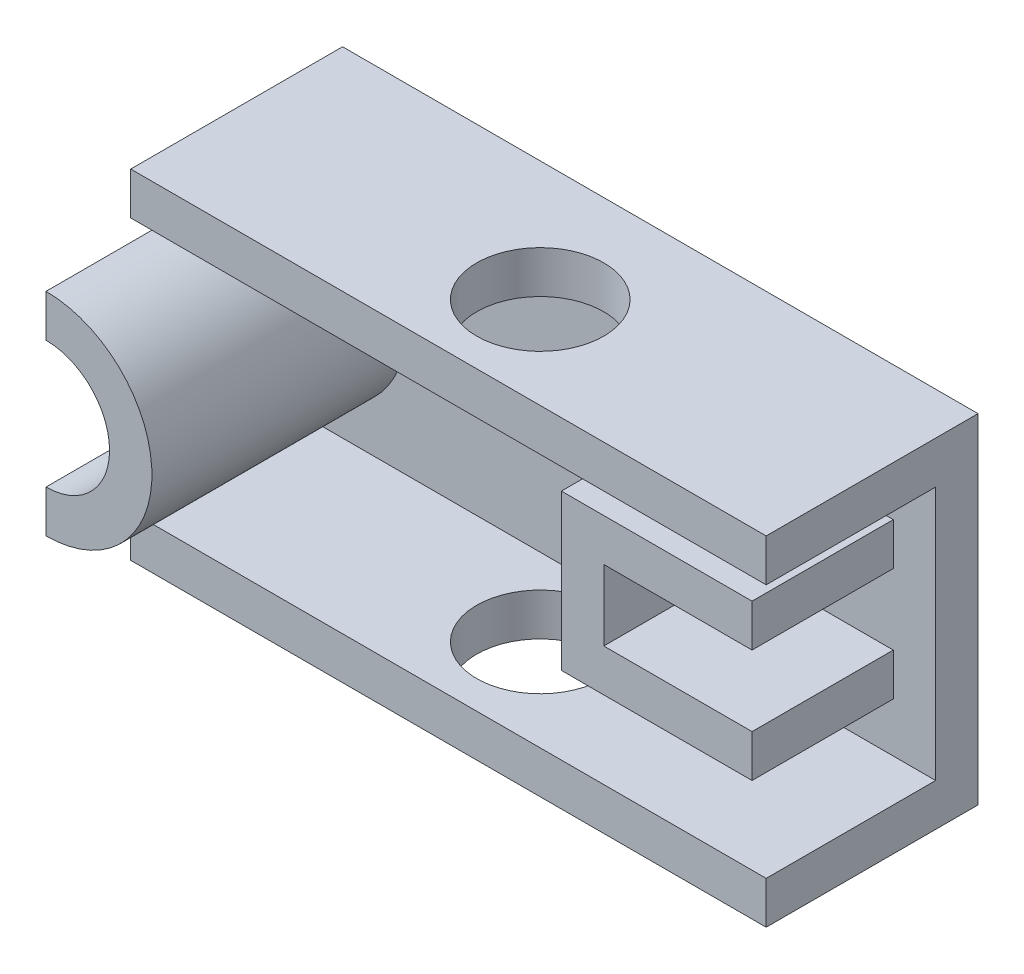
ISO-10303-21;
HEADER;
FILE_DESCRIPTION(('STEP AP214'),'2;1');
FILE_NAME('part.step','',(''),(''),'','','');
FILE_SCHEMA(('AUTOMOTIVE_DESIGN { 1 0 10303 214 1 1 1 1 }'));
ENDSEC;
DATA;
#1=APPLICATION_CONTEXT('core data for automotive mechanical design processes');
#2=APPLICATION_PROTOCOL_DEFINITION('international standard','automotive_design',2000,#1);
#3=PRODUCT_CONTEXT('',#1,'mechanical');
#4=PRODUCT('Part','Part','',(#3));
#5=PRODUCT_RELATED_PRODUCT_CATEGORY('part','',(#4));
#6=PRODUCT_DEFINITION_FORMATION('','',#4);
#7=PRODUCT_DEFINITION_CONTEXT('part definition',#1,'design');
#8=PRODUCT_DEFINITION('design','',#6,#7);
#9=PRODUCT_DEFINITION_SHAPE('','',#8);
#10=(LENGTH_UNIT() NAMED_UNIT(*) SI_UNIT(.MILLI.,.METRE.));
#11=(NAMED_UNIT(*) PLANE_ANGLE_UNIT() SI_UNIT($,.RADIAN.));
#12=(NAMED_UNIT(*) SI_UNIT($,.STERADIAN.) SOLID_ANGLE_UNIT());
#13=UNCERTAINTY_MEASURE_WITH_UNIT(LENGTH_MEASURE(1.E-05),#10,'distance_accuracy_value','');
#14=(GEOMETRIC_REPRESENTATION_CONTEXT(3) GLOBAL_UNCERTAINTY_ASSIGNED_CONTEXT((#13)) GLOBAL_UNIT_ASSIGNED_CONTEXT((#10,
#11,#12)) REPRESENTATION_CONTEXT('',''));
#15=CARTESIAN_POINT('',(0.,0.,0.));
#16=DIRECTION('',(0.,0.,1.));
#17=DIRECTION('',(1.,0.,0.));
#18=AXIS2_PLACEMENT_3D('',#15,#16,#17);
#19=CARTESIAN_POINT('',(0.,0.,6.));
#20=DIRECTION('',(0.,0.,1.));
#21=DIRECTION('',(1.,0.,0.));
#22=AXIS2_PLACEMENT_3D('',#19,#20,#21);
#23=PLANE('',#22);
#24=DIRECTION('',(0.,-1.,0.));
#25=VECTOR('',#24,1.);
#26=CARTESIAN_POINT('',(0.,42.,6.));
#27=LINE('',#26,#25);
#28=CARTESIAN_POINT('',(0.,42.,6.));
#29=VERTEX_POINT('',#28);
#30=CARTESIAN_POINT('',(0.,39.,6.));
#31=VERTEX_POINT('',#30);
#32=EDGE_CURVE('E258',#29,#31,#27,.T.);
#33=ORIENTED_EDGE('',*,*,#32,.T.);
#34=CARTESIAN_POINT('',(0.,24.,6.));
#35=DIRECTION('',(0.,0.,1.));
#36=DIRECTION('',(1.,0.,0.));
#37=AXIS2_PLACEMENT_3D('',#34,#35,#36);
#38=CIRCLE('',#37,15.);
#39=CARTESIAN_POINT('',(0.,9.,6.));
#40=VERTEX_POINT('',#39);
#41=EDGE_CURVE('E233',#40,#31,#38,.T.);
#42=ORIENTED_EDGE('',*,*,#41,.F.);
#43=CARTESIAN_POINT('',(0.,6.,6.));
#44=VERTEX_POINT('',#43);
#45=EDGE_CURVE('E259',#40,#44,#27,.T.);
#46=ORIENTED_EDGE('',*,*,#45,.T.);
#47=DIRECTION('',(1.,0.,0.));
#48=VECTOR('',#47,1.);
#49=CARTESIAN_POINT('',(6.00000000000003,6.,6.));
#50=LINE('',#49,#48);
#51=CARTESIAN_POINT('',(90.,6.,6.));
#52=VERTEX_POINT('',#51);
#53=EDGE_CURVE('E268',#44,#52,#50,.T.);
#54=ORIENTED_EDGE('',*,*,#53,.T.);
#55=DIRECTION('',(0.,1.,0.));
#56=VECTOR('',#55,1.);
#57=CARTESIAN_POINT('',(90.,6.,6.));
#58=LINE('',#57,#56);
#59=CARTESIAN_POINT('',(90.,42.,6.));
#60=VERTEX_POINT('',#59);
#61=EDGE_CURVE('E248',#52,#60,#58,.T.);
#62=ORIENTED_EDGE('',*,*,#61,.T.);
#63=DIRECTION('',(-1.,0.,0.));
#64=VECTOR('',#63,1.);
#65=CARTESIAN_POINT('',(84.,42.,6.));
#66=LINE('',#65,#64);
#67=EDGE_CURVE('E270',#60,#29,#66,.T.);
#68=ORIENTED_EDGE('',*,*,#67,.T.);
#69=EDGE_LOOP('',(#33,#42,#46,#54,#62,#68));
#70=FACE_BOUND('',#69,.T.);
#71=DIRECTION('',(0.,-1.,0.));
#72=VECTOR('',#71,1.);
#73=CARTESIAN_POINT('',(57.,35.,6.));
#74=LINE('',#73,#72);
#75=CARTESIAN_POINT('',(57.,35.,6.));
#76=VERTEX_POINT('',#75);
#77=CARTESIAN_POINT('',(57.,13.,6.));
#78=VERTEX_POINT('',#77);
#79=EDGE_CURVE('E689',#76,#78,#74,.T.);
#80=ORIENTED_EDGE('',*,*,#79,.F.);
#81=DIRECTION('',(-1.,0.,0.));
#82=VECTOR('',#81,1.);
#83=CARTESIAN_POINT('',(84.,35.,6.));
#84=LINE('',#83,#82);
#85=CARTESIAN_POINT('',(84.,35.,6.));
#86=VERTEX_POINT('',#85);
#87=EDGE_CURVE('E203',#86,#76,#84,.T.);
#88=ORIENTED_EDGE('',*,*,#87,.F.);
#89=DIRECTION('',(0.,1.,0.));
#90=VECTOR('',#89,1.);
#91=CARTESIAN_POINT('',(84.,35.,6.));
#92=LINE('',#91,#90);
#93=CARTESIAN_POINT('',(84.,29.,6.));
#94=VERTEX_POINT('',#93);
#95=EDGE_CURVE('E202',#94,#86,#92,.T.);
#96=ORIENTED_EDGE('',*,*,#95,.F.);
#97=DIRECTION('',(1.,0.,0.));
#98=VECTOR('',#97,1.);
#99=CARTESIAN_POINT('',(84.,29.,6.));
#100=LINE('',#99,#98);
#101=CARTESIAN_POINT('',(63.,29.,6.));
#102=VERTEX_POINT('',#101);
#103=EDGE_CURVE('E684',#102,#94,#100,.T.);
#104=ORIENTED_EDGE('',*,*,#103,.F.);
#105=DIRECTION('',(0.,1.,0.));
#106=VECTOR('',#105,1.);
#107=CARTESIAN_POINT('',(63.,19.,6.));
#108=LINE('',#107,#106);
#109=CARTESIAN_POINT('',(63.,19.,6.));
#110=VERTEX_POINT('',#109);
#111=EDGE_CURVE('E701',#110,#102,#108,.T.);
#112=ORIENTED_EDGE('',*,*,#111,.F.);
#113=DIRECTION('',(-1.,0.,0.));
#114=VECTOR('',#113,1.);
#115=CARTESIAN_POINT('',(84.,19.,6.));
#116=LINE('',#115,#114);
#117=CARTESIAN_POINT('',(84.,19.,6.));
#118=VERTEX_POINT('',#117);
#119=EDGE_CURVE('E697',#118,#110,#116,.T.);
#120=ORIENTED_EDGE('',*,*,#119,.F.);
#121=DIRECTION('',(0.,1.,0.));
#122=VECTOR('',#121,1.);
#123=CARTESIAN_POINT('',(84.,19.,6.));
#124=LINE('',#123,#122);
#125=CARTESIAN_POINT('',(84.,13.,6.));
#126=VERTEX_POINT('',#125);
#127=EDGE_CURVE('E700',#126,#118,#124,.T.);
#128=ORIENTED_EDGE('',*,*,#127,.F.);
#129=DIRECTION('',(1.,0.,0.));
#130=VECTOR('',#129,1.);
#131=CARTESIAN_POINT('',(57.,13.,6.));
#132=LINE('',#131,#130);
#133=EDGE_CURVE('E691',#78,#126,#132,.T.);
#134=ORIENTED_EDGE('',*,*,#133,.F.);
#135=EDGE_LOOP('',(#80,#88,#96,#104,#112,#120,#128,#134));
#136=FACE_BOUND('',#135,.T.);
#137=ADVANCED_FACE('F44',(#70,#136),#23,.T.);
#138=CARTESIAN_POINT('',(0.,48.,30.));
#139=DIRECTION('',(1.,0.,0.));
#140=DIRECTION('',(0.,0.,-1.));
#141=AXIS2_PLACEMENT_3D('',#138,#139,#140);
#142=PLANE('',#141);
#143=DIRECTION('',(0.,-1.,0.));
#144=VECTOR('',#143,1.);
#145=CARTESIAN_POINT('',(0.,48.,0.));
#146=LINE('',#145,#144);
#147=CARTESIAN_POINT('',(0.,48.,0.));
#148=VERTEX_POINT('',#147);
#149=CARTESIAN_POINT('',(0.,33.,0.));
#150=VERTEX_POINT('',#149);
#151=EDGE_CURVE('E286',#148,#150,#146,.T.);
#152=ORIENTED_EDGE('',*,*,#151,.T.);
#153=DIRECTION('',(0.,0.,1.));
#154=VECTOR('',#153,1.);
#155=CARTESIAN_POINT('',(0.,33.,0.));
#156=LINE('',#155,#154);
#157=CARTESIAN_POINT('',(0.,33.,42.));
#158=VERTEX_POINT('',#157);
#159=EDGE_CURVE('E226',#150,#158,#156,.T.);
#160=ORIENTED_EDGE('',*,*,#159,.T.);
#161=DIRECTION('',(0.,-1.,0.));
#162=VECTOR('',#161,1.);
#163=CARTESIAN_POINT('',(0.,39.,42.));
#164=LINE('',#163,#162);
#165=CARTESIAN_POINT('',(0.,39.,42.));
#166=VERTEX_POINT('',#165);
#167=EDGE_CURVE('E238',#166,#158,#164,.T.);
#168=ORIENTED_EDGE('',*,*,#167,.F.);
#169=DIRECTION('',(0.,0.,-1.));
#170=VECTOR('',#169,1.);
#171=CARTESIAN_POINT('',(0.,39.,42.));
#172=LINE('',#171,#170);
#173=EDGE_CURVE('E246',#166,#31,#172,.T.);
#174=ORIENTED_EDGE('',*,*,#173,.T.);
#175=ORIENTED_EDGE('',*,*,#32,.F.);
#176=DIRECTION('',(0.,0.,1.));
#177=VECTOR('',#176,1.);
#178=CARTESIAN_POINT('',(0.,42.,6.));
#179=LINE('',#178,#177);
#180=CARTESIAN_POINT('',(0.,42.,30.));
#181=VERTEX_POINT('',#180);
#182=EDGE_CURVE('E263',#29,#181,#179,.T.);
#183=ORIENTED_EDGE('',*,*,#182,.T.);
#184=DIRECTION('',(0.,-1.,0.));
#185=VECTOR('',#184,1.);
#186=CARTESIAN_POINT('',(0.,48.,30.));
#187=LINE('',#186,#185);
#188=CARTESIAN_POINT('',(0.,48.,30.));
#189=VERTEX_POINT('',#188);
#190=EDGE_CURVE('E279',#189,#181,#187,.T.);
#191=ORIENTED_EDGE('',*,*,#190,.F.);
#192=DIRECTION('',(0.,0.,-1.));
#193=VECTOR('',#192,1.);
#194=CARTESIAN_POINT('',(0.,48.,30.));
#195=LINE('',#194,#193);
#196=EDGE_CURVE('E290',#189,#148,#195,.T.);
#197=ORIENTED_EDGE('',*,*,#196,.T.);
#198=EDGE_LOOP('',(#152,#160,#168,#174,#175,#183,#191,#197));
#199=FACE_BOUND('',#198,.T.);
#200=ADVANCED_FACE('F323',(#199),#142,.F.);
#201=CARTESIAN_POINT('',(0.,0.,30.));
#202=DIRECTION('',(0.,0.,1.));
#203=DIRECTION('',(1.,0.,0.));
#204=AXIS2_PLACEMENT_3D('',#201,#202,#203);
#205=PLANE('',#204);
#206=DIRECTION('',(-1.,0.,0.));
#207=VECTOR('',#206,1.);
#208=CARTESIAN_POINT('',(84.,42.,30.));
#209=LINE('',#208,#207);
#210=CARTESIAN_POINT('',(90.,42.,30.));
#211=VERTEX_POINT('',#210);
#212=EDGE_CURVE('E261',#211,#181,#209,.T.);
#213=ORIENTED_EDGE('',*,*,#212,.F.);
#214=DIRECTION('',(0.,1.,0.));
#215=VECTOR('',#214,1.);
#216=CARTESIAN_POINT('',(90.,0.,30.));
#217=LINE('',#216,#215);
#218=CARTESIAN_POINT('',(90.,48.,30.));
#219=VERTEX_POINT('',#218);
#220=EDGE_CURVE('E284',#211,#219,#217,.T.);
#221=ORIENTED_EDGE('',*,*,#220,.T.);
#222=DIRECTION('',(-1.,0.,0.));
#223=VECTOR('',#222,1.);
#224=CARTESIAN_POINT('',(90.,48.,30.));
#225=LINE('',#224,#223);
#226=EDGE_CURVE('E287',#219,#189,#225,.T.);
#227=ORIENTED_EDGE('',*,*,#226,.T.);
#228=ORIENTED_EDGE('',*,*,#190,.T.);
#229=EDGE_LOOP('',(#213,#221,#227,#228));
#230=FACE_BOUND('',#229,.T.);
#231=ADVANCED_FACE('F327',(#230),#205,.T.);
#232=CARTESIAN_POINT('',(0.,15.,42.));
#233=VERTEX_POINT('',#232);
#234=CARTESIAN_POINT('',(0.,9.,42.));
#235=VERTEX_POINT('',#234);
#236=EDGE_CURVE('E240',#233,#235,#164,.T.);
#237=ORIENTED_EDGE('',*,*,#236,.F.);
#238=DIRECTION('',(0.,0.,1.));
#239=VECTOR('',#238,1.);
#240=CARTESIAN_POINT('',(0.,15.,0.));
#241=LINE('',#240,#239);
#242=CARTESIAN_POINT('',(0.,15.,0.));
#243=VERTEX_POINT('',#242);
#244=EDGE_CURVE('E67',#243,#233,#241,.T.);
#245=ORIENTED_EDGE('',*,*,#244,.F.);
#246=CARTESIAN_POINT('',(0.,0.,0.));
#247=VERTEX_POINT('',#246);
#248=EDGE_CURVE('E271',#243,#247,#146,.T.);
#249=ORIENTED_EDGE('',*,*,#248,.T.);
#250=DIRECTION('',(0.,0.,-1.));
#251=VECTOR('',#250,1.);
#252=CARTESIAN_POINT('',(0.,0.,30.));
#253=LINE('',#252,#251);
#254=CARTESIAN_POINT('',(0.,0.,30.));
#255=VERTEX_POINT('',#254);
#256=EDGE_CURVE('E11',#255,#247,#253,.T.);
#257=ORIENTED_EDGE('',*,*,#256,.F.);
#258=CARTESIAN_POINT('',(0.,6.,30.));
#259=VERTEX_POINT('',#258);
#260=EDGE_CURVE('E277',#259,#255,#187,.T.);
#261=ORIENTED_EDGE('',*,*,#260,.F.);
#262=DIRECTION('',(0.,0.,1.));
#263=VECTOR('',#262,1.);
#264=CARTESIAN_POINT('',(0.,6.,6.));
#265=LINE('',#264,#263);
#266=EDGE_CURVE('E264',#44,#259,#265,.T.);
#267=ORIENTED_EDGE('',*,*,#266,.F.);
#268=ORIENTED_EDGE('',*,*,#45,.F.);
#269=DIRECTION('',(0.,0.,-1.));
#270=VECTOR('',#269,1.);
#271=CARTESIAN_POINT('',(0.,9.,42.));
#272=LINE('',#271,#270);
#273=EDGE_CURVE('E241',#235,#40,#272,.T.);
#274=ORIENTED_EDGE('',*,*,#273,.F.);
#275=EDGE_LOOP('',(#237,#245,#249,#257,#261,#267,#268,#274));
#276=FACE_BOUND('',#275,.T.);
#277=ADVANCED_FACE('F50',(#276),#142,.F.);
#278=CARTESIAN_POINT('',(0.,0.,30.));
#279=DIRECTION('',(0.,1.,0.));
#280=DIRECTION('',(0.,0.,1.));
#281=AXIS2_PLACEMENT_3D('',#278,#279,#280);
#282=PLANE('',#281);
#283=CARTESIAN_POINT('',(45.,0.,17.));
#284=DIRECTION('',(0.,-1.,0.));
#285=DIRECTION('',(0.,0.,-1.));
#286=AXIS2_PLACEMENT_3D('',#283,#284,#285);
#287=CIRCLE('',#286,9.);
#288=CARTESIAN_POINT('',(45.,0.,8.));
#289=VERTEX_POINT('',#288);
#290=EDGE_CURVE('E219',#289,#289,#287,.T.);
#291=ORIENTED_EDGE('',*,*,#290,.F.);
#292=EDGE_LOOP('',(#291));
#293=FACE_BOUND('',#292,.T.);
#294=DIRECTION('',(1.,0.,0.));
#295=VECTOR('',#294,1.);
#296=CARTESIAN_POINT('',(0.,0.,0.));
#297=LINE('',#296,#295);
#298=CARTESIAN_POINT('',(90.,0.,0.));
#299=VERTEX_POINT('',#298);
#300=EDGE_CURVE('E292',#247,#299,#297,.T.);
#301=ORIENTED_EDGE('',*,*,#300,.T.);
#302=DIRECTION('',(0.,0.,-1.));
#303=VECTOR('',#302,1.);
#304=CARTESIAN_POINT('',(90.,0.,30.));
#305=LINE('',#304,#303);
#306=CARTESIAN_POINT('',(90.,0.,30.));
#307=VERTEX_POINT('',#306);
#308=EDGE_CURVE('E52',#307,#299,#305,.T.);
#309=ORIENTED_EDGE('',*,*,#308,.F.);
#310=DIRECTION('',(1.,0.,0.));
#311=VECTOR('',#310,1.);
#312=CARTESIAN_POINT('',(0.,0.,30.));
#313=LINE('',#312,#311);
#314=EDGE_CURVE('E278',#255,#307,#313,.T.);
#315=ORIENTED_EDGE('',*,*,#314,.F.);
#316=ORIENTED_EDGE('',*,*,#256,.T.);
#317=EDGE_LOOP('',(#301,#309,#315,#316));
#318=FACE_BOUND('',#317,.T.);
#319=ADVANCED_FACE('F342',(#293,#318),#282,.F.);
#320=CARTESIAN_POINT('',(90.,0.,30.));
#321=DIRECTION('',(-1.,0.,0.));
#322=DIRECTION('',(0.,0.,1.));
#323=AXIS2_PLACEMENT_3D('',#320,#321,#322);
#324=PLANE('',#323);
#325=ORIENTED_EDGE('',*,*,#220,.F.);
#326=DIRECTION('',(0.,0.,1.));
#327=VECTOR('',#326,1.);
#328=CARTESIAN_POINT('',(90.,42.,6.));
#329=LINE('',#328,#327);
#330=EDGE_CURVE('E254',#60,#211,#329,.T.);
#331=ORIENTED_EDGE('',*,*,#330,.F.);
#332=ORIENTED_EDGE('',*,*,#61,.F.);
#333=DIRECTION('',(0.,0.,1.));
#334=VECTOR('',#333,1.);
#335=CARTESIAN_POINT('',(90.,6.,6.));
#336=LINE('',#335,#334);
#337=CARTESIAN_POINT('',(90.,6.,30.));
#338=VERTEX_POINT('',#337);
#339=EDGE_CURVE('E255',#52,#338,#336,.T.);
#340=ORIENTED_EDGE('',*,*,#339,.T.);
#341=EDGE_CURVE('E282',#307,#338,#217,.T.);
#342=ORIENTED_EDGE('',*,*,#341,.F.);
#343=ORIENTED_EDGE('',*,*,#308,.T.);
#344=DIRECTION('',(0.,1.,0.));
#345=VECTOR('',#344,1.);
#346=CARTESIAN_POINT('',(90.,0.,0.));
#347=LINE('',#346,#345);
#348=CARTESIAN_POINT('',(90.,48.,0.));
#349=VERTEX_POINT('',#348);
#350=EDGE_CURVE('E295',#299,#349,#347,.T.);
#351=ORIENTED_EDGE('',*,*,#350,.T.);
#352=DIRECTION('',(0.,0.,-1.));
#353=VECTOR('',#352,1.);
#354=CARTESIAN_POINT('',(90.,48.,30.));
#355=LINE('',#354,#353);
#356=EDGE_CURVE('E297',#219,#349,#355,.T.);
#357=ORIENTED_EDGE('',*,*,#356,.F.);
#358=EDGE_LOOP('',(#325,#331,#332,#340,#342,#343,#351,#357));
#359=FACE_BOUND('',#358,.T.);
#360=ADVANCED_FACE('F308',(#359),#324,.F.);
#361=CARTESIAN_POINT('',(90.,48.,30.));
#362=DIRECTION('',(0.,-1.,0.));
#363=DIRECTION('',(0.,0.,-1.));
#364=AXIS2_PLACEMENT_3D('',#361,#362,#363);
#365=PLANE('',#364);
#366=CARTESIAN_POINT('',(45.,48.,17.));
#367=DIRECTION('',(0.,1.,0.));
#368=DIRECTION('',(0.,0.,1.));
#369=AXIS2_PLACEMENT_3D('',#366,#367,#368);
#370=CIRCLE('',#369,9.);
#371=CARTESIAN_POINT('',(45.,48.,26.));
#372=VERTEX_POINT('',#371);
#373=EDGE_CURVE('E210',#372,#372,#370,.T.);
#374=ORIENTED_EDGE('',*,*,#373,.F.);
#375=EDGE_LOOP('',(#374));
#376=FACE_BOUND('',#375,.T.);
#377=DIRECTION('',(-1.,0.,0.));
#378=VECTOR('',#377,1.);
#379=CARTESIAN_POINT('',(90.,48.,0.));
#380=LINE('',#379,#378);
#381=EDGE_CURVE('E298',#349,#148,#380,.T.);
#382=ORIENTED_EDGE('',*,*,#381,.T.);
#383=ORIENTED_EDGE('',*,*,#196,.F.);
#384=ORIENTED_EDGE('',*,*,#226,.F.);
#385=ORIENTED_EDGE('',*,*,#356,.T.);
#386=EDGE_LOOP('',(#382,#383,#384,#385));
#387=FACE_BOUND('',#386,.T.);
#388=ADVANCED_FACE('F318',(#376,#387),#365,.F.);
#389=ORIENTED_EDGE('',*,*,#341,.T.);
#390=DIRECTION('',(1.,0.,0.));
#391=VECTOR('',#390,1.);
#392=CARTESIAN_POINT('',(6.00000000000003,6.,30.));
#393=LINE('',#392,#391);
#394=EDGE_CURVE('E272',#259,#338,#393,.T.);
#395=ORIENTED_EDGE('',*,*,#394,.F.);
#396=ORIENTED_EDGE('',*,*,#260,.T.);
#397=ORIENTED_EDGE('',*,*,#314,.T.);
#398=EDGE_LOOP('',(#389,#395,#396,#397));
#399=FACE_BOUND('',#398,.T.);
#400=ADVANCED_FACE('F341',(#399),#205,.T.);
#401=CARTESIAN_POINT('',(0.,0.,0.));
#402=DIRECTION('',(0.,0.,1.));
#403=DIRECTION('',(1.,0.,0.));
#404=AXIS2_PLACEMENT_3D('',#401,#402,#403);
#405=PLANE('',#404);
#406=ORIENTED_EDGE('',*,*,#248,.F.);
#407=CARTESIAN_POINT('',(0.,24.,0.));
#408=DIRECTION('',(0.,0.,1.));
#409=DIRECTION('',(1.,0.,0.));
#410=AXIS2_PLACEMENT_3D('',#407,#408,#409);
#411=CIRCLE('',#410,9.);
#412=EDGE_CURVE('E223',#243,#150,#411,.T.);
#413=ORIENTED_EDGE('',*,*,#412,.T.);
#414=ORIENTED_EDGE('',*,*,#151,.F.);
#415=ORIENTED_EDGE('',*,*,#381,.F.);
#416=ORIENTED_EDGE('',*,*,#350,.F.);
#417=ORIENTED_EDGE('',*,*,#300,.F.);
#418=EDGE_LOOP('',(#406,#413,#414,#415,#416,#417));
#419=FACE_BOUND('',#418,.T.);
#420=ADVANCED_FACE('F317',(#419),#405,.F.);
#421=CARTESIAN_POINT('',(84.,42.,6.));
#422=DIRECTION('',(0.,1.,0.));
#423=DIRECTION('',(0.,0.,1.));
#424=AXIS2_PLACEMENT_3D('',#421,#422,#423);
#425=PLANE('',#424);
#426=CARTESIAN_POINT('',(45.,42.,17.));
#427=DIRECTION('',(0.,1.,0.));
#428=DIRECTION('',(0.,0.,1.));
#429=AXIS2_PLACEMENT_3D('',#426,#427,#428);
#430=CIRCLE('',#429,9.);
#431=CARTESIAN_POINT('',(45.,42.,26.));
#432=VERTEX_POINT('',#431);
#433=EDGE_CURVE('E208',#432,#432,#430,.T.);
#434=ORIENTED_EDGE('',*,*,#433,.T.);
#435=EDGE_LOOP('',(#434));
#436=FACE_BOUND('',#435,.T.);
#437=ORIENTED_EDGE('',*,*,#212,.T.);
#438=ORIENTED_EDGE('',*,*,#182,.F.);
#439=ORIENTED_EDGE('',*,*,#67,.F.);
#440=ORIENTED_EDGE('',*,*,#330,.T.);
#441=EDGE_LOOP('',(#437,#438,#439,#440));
#442=FACE_BOUND('',#441,.T.);
#443=ADVANCED_FACE('F334',(#436,#442),#425,.F.);
#444=CARTESIAN_POINT('',(6.00000000000003,6.,6.));
#445=DIRECTION('',(0.,-1.,0.));
#446=DIRECTION('',(0.,0.,-1.));
#447=AXIS2_PLACEMENT_3D('',#444,#445,#446);
#448=PLANE('',#447);
#449=CARTESIAN_POINT('',(45.,6.,17.));
#450=DIRECTION('',(0.,-1.,0.));
#451=DIRECTION('',(0.,0.,-1.));
#452=AXIS2_PLACEMENT_3D('',#449,#450,#451);
#453=CIRCLE('',#452,9.);
#454=CARTESIAN_POINT('',(45.,6.,8.));
#455=VERTEX_POINT('',#454);
#456=EDGE_CURVE('E220',#455,#455,#453,.T.);
#457=ORIENTED_EDGE('',*,*,#456,.T.);
#458=EDGE_LOOP('',(#457));
#459=FACE_BOUND('',#458,.T.);
#460=ORIENTED_EDGE('',*,*,#394,.T.);
#461=ORIENTED_EDGE('',*,*,#339,.F.);
#462=ORIENTED_EDGE('',*,*,#53,.F.);
#463=ORIENTED_EDGE('',*,*,#266,.T.);
#464=EDGE_LOOP('',(#460,#461,#462,#463));
#465=FACE_BOUND('',#464,.T.);
#466=ADVANCED_FACE('F338',(#459,#465),#448,.F.);
#467=CARTESIAN_POINT('',(0.,24.,42.));
#468=DIRECTION('',(0.,0.,-1.));
#469=DIRECTION('',(-1.,0.,0.));
#470=AXIS2_PLACEMENT_3D('',#467,#468,#469);
#471=CYLINDRICAL_SURFACE('',#470,15.);
#472=ORIENTED_EDGE('',*,*,#41,.T.);
#473=ORIENTED_EDGE('',*,*,#173,.F.);
#474=CARTESIAN_POINT('',(0.,24.,42.));
#475=DIRECTION('',(0.,0.,1.));
#476=DIRECTION('',(1.,0.,0.));
#477=AXIS2_PLACEMENT_3D('',#474,#475,#476);
#478=CIRCLE('',#477,15.);
#479=EDGE_CURVE('E234',#235,#166,#478,.T.);
#480=ORIENTED_EDGE('',*,*,#479,.F.);
#481=ORIENTED_EDGE('',*,*,#273,.T.);
#482=EDGE_LOOP('',(#472,#473,#480,#481));
#483=FACE_BOUND('',#482,.T.);
#484=ADVANCED_FACE('F353',(#483),#471,.T.);
#485=CARTESIAN_POINT('',(0.,24.,42.));
#486=DIRECTION('',(0.,0.,1.));
#487=DIRECTION('',(1.,0.,0.));
#488=AXIS2_PLACEMENT_3D('',#485,#486,#487);
#489=PLANE('',#488);
#490=CARTESIAN_POINT('',(0.,24.,42.));
#491=DIRECTION('',(0.,0.,1.));
#492=DIRECTION('',(1.,0.,0.));
#493=AXIS2_PLACEMENT_3D('',#490,#491,#492);
#494=CIRCLE('',#493,9.);
#495=EDGE_CURVE('E224',#233,#158,#494,.T.);
#496=ORIENTED_EDGE('',*,*,#495,.F.);
#497=ORIENTED_EDGE('',*,*,#236,.T.);
#498=ORIENTED_EDGE('',*,*,#479,.T.);
#499=ORIENTED_EDGE('',*,*,#167,.T.);
#500=EDGE_LOOP('',(#496,#497,#498,#499));
#501=FACE_BOUND('',#500,.T.);
#502=ADVANCED_FACE('F346',(#501),#489,.T.);
#503=CARTESIAN_POINT('',(0.,24.,0.));
#504=DIRECTION('',(0.,0.,1.));
#505=DIRECTION('',(1.,0.,0.));
#506=AXIS2_PLACEMENT_3D('',#503,#504,#505);
#507=CYLINDRICAL_SURFACE('',#506,9.);
#508=ORIENTED_EDGE('',*,*,#495,.T.);
#509=ORIENTED_EDGE('',*,*,#159,.F.);
#510=ORIENTED_EDGE('',*,*,#412,.F.);
#511=ORIENTED_EDGE('',*,*,#244,.T.);
#512=EDGE_LOOP('',(#508,#509,#510,#511));
#513=FACE_BOUND('',#512,.T.);
#514=ADVANCED_FACE('F347',(#513),#507,.F.);
#515=CARTESIAN_POINT('',(45.,6.,17.));
#516=DIRECTION('',(0.,-1.,0.));
#517=DIRECTION('',(0.,0.,-1.));
#518=AXIS2_PLACEMENT_3D('',#515,#516,#517);
#519=CYLINDRICAL_SURFACE('',#518,9.);
#520=ORIENTED_EDGE('',*,*,#456,.F.);
#521=EDGE_LOOP('',(#520));
#522=FACE_BOUND('',#521,.T.);
#523=ORIENTED_EDGE('',*,*,#290,.T.);
#524=EDGE_LOOP('',(#523));
#525=FACE_BOUND('',#524,.T.);
#526=ADVANCED_FACE('F394',(#522,#525),#519,.F.);
#527=CARTESIAN_POINT('',(45.,42.,17.));
#528=DIRECTION('',(0.,1.,0.));
#529=DIRECTION('',(0.,0.,1.));
#530=AXIS2_PLACEMENT_3D('',#527,#528,#529);
#531=CYLINDRICAL_SURFACE('',#530,9.);
#532=ORIENTED_EDGE('',*,*,#433,.F.);
#533=EDGE_LOOP('',(#532));
#534=FACE_BOUND('',#533,.T.);
#535=ORIENTED_EDGE('',*,*,#373,.T.);
#536=EDGE_LOOP('',(#535));
#537=FACE_BOUND('',#536,.T.);
#538=ADVANCED_FACE('F395',(#534,#537),#531,.F.);
#539=CARTESIAN_POINT('',(84.,35.,26.));
#540=DIRECTION('',(0.,-1.,0.));
#541=DIRECTION('',(0.,0.,-1.));
#542=AXIS2_PLACEMENT_3D('',#539,#540,#541);
#543=PLANE('',#542);
#544=ORIENTED_EDGE('',*,*,#87,.T.);
#545=DIRECTION('',(0.,0.,-1.));
#546=VECTOR('',#545,1.);
#547=CARTESIAN_POINT('',(57.,35.,26.));
#548=LINE('',#547,#546);
#549=CARTESIAN_POINT('',(57.,35.,26.));
#550=VERTEX_POINT('',#549);
#551=EDGE_CURVE('E187',#550,#76,#548,.T.);
#552=ORIENTED_EDGE('',*,*,#551,.F.);
#553=DIRECTION('',(-1.,0.,0.));
#554=VECTOR('',#553,1.);
#555=CARTESIAN_POINT('',(84.,35.,26.));
#556=LINE('',#555,#554);
#557=CARTESIAN_POINT('',(84.,35.,26.));
#558=VERTEX_POINT('',#557);
#559=EDGE_CURVE('E195',#558,#550,#556,.T.);
#560=ORIENTED_EDGE('',*,*,#559,.F.);
#561=DIRECTION('',(0.,0.,-1.));
#562=VECTOR('',#561,1.);
#563=CARTESIAN_POINT('',(84.,35.,26.));
#564=LINE('',#563,#562);
#565=EDGE_CURVE('E681',#558,#86,#564,.T.);
#566=ORIENTED_EDGE('',*,*,#565,.T.);
#567=EDGE_LOOP('',(#544,#552,#560,#566));
#568=FACE_BOUND('',#567,.T.);
#569=ADVANCED_FACE('F205',(#568),#543,.F.);
#570=CARTESIAN_POINT('',(57.,35.,26.));
#571=DIRECTION('',(1.,0.,0.));
#572=DIRECTION('',(0.,0.,-1.));
#573=AXIS2_PLACEMENT_3D('',#570,#571,#572);
#574=PLANE('',#573);
#575=ORIENTED_EDGE('',*,*,#79,.T.);
#576=DIRECTION('',(0.,0.,-1.));
#577=VECTOR('',#576,1.);
#578=CARTESIAN_POINT('',(57.,13.,26.));
#579=LINE('',#578,#577);
#580=CARTESIAN_POINT('',(57.,13.,26.));
#581=VERTEX_POINT('',#580);
#582=EDGE_CURVE('E186',#581,#78,#579,.T.);
#583=ORIENTED_EDGE('',*,*,#582,.F.);
#584=DIRECTION('',(0.,-1.,0.));
#585=VECTOR('',#584,1.);
#586=CARTESIAN_POINT('',(57.,35.,26.));
#587=LINE('',#586,#585);
#588=EDGE_CURVE('E185',#550,#581,#587,.T.);
#589=ORIENTED_EDGE('',*,*,#588,.F.);
#590=ORIENTED_EDGE('',*,*,#551,.T.);
#591=EDGE_LOOP('',(#575,#583,#589,#590));
#592=FACE_BOUND('',#591,.T.);
#593=ADVANCED_FACE('F183',(#592),#574,.F.);
#594=CARTESIAN_POINT('',(57.,13.,26.));
#595=DIRECTION('',(0.,1.,0.));
#596=DIRECTION('',(0.,0.,1.));
#597=AXIS2_PLACEMENT_3D('',#594,#595,#596);
#598=PLANE('',#597);
#599=ORIENTED_EDGE('',*,*,#133,.T.);
#600=DIRECTION('',(0.,0.,-1.));
#601=VECTOR('',#600,1.);
#602=CARTESIAN_POINT('',(84.,13.,26.));
#603=LINE('',#602,#601);
#604=CARTESIAN_POINT('',(84.,13.,26.));
#605=VERTEX_POINT('',#604);
#606=EDGE_CURVE('E211',#605,#126,#603,.T.);
#607=ORIENTED_EDGE('',*,*,#606,.F.);
#608=DIRECTION('',(1.,0.,0.));
#609=VECTOR('',#608,1.);
#610=CARTESIAN_POINT('',(57.,13.,26.));
#611=LINE('',#610,#609);
#612=EDGE_CURVE('E191',#581,#605,#611,.T.);
#613=ORIENTED_EDGE('',*,*,#612,.F.);
#614=ORIENTED_EDGE('',*,*,#582,.T.);
#615=EDGE_LOOP('',(#599,#607,#613,#614));
#616=FACE_BOUND('',#615,.T.);
#617=ADVANCED_FACE('F407',(#616),#598,.F.);
#618=CARTESIAN_POINT('',(84.,19.,26.));
#619=DIRECTION('',(-1.,0.,0.));
#620=DIRECTION('',(0.,0.,1.));
#621=AXIS2_PLACEMENT_3D('',#618,#619,#620);
#622=PLANE('',#621);
#623=ORIENTED_EDGE('',*,*,#127,.T.);
#624=DIRECTION('',(0.,0.,-1.));
#625=VECTOR('',#624,1.);
#626=CARTESIAN_POINT('',(84.,19.,26.));
#627=LINE('',#626,#625);
#628=CARTESIAN_POINT('',(84.,19.,26.));
#629=VERTEX_POINT('',#628);
#630=EDGE_CURVE('E714',#629,#118,#627,.T.);
#631=ORIENTED_EDGE('',*,*,#630,.F.);
#632=DIRECTION('',(0.,1.,0.));
#633=VECTOR('',#632,1.);
#634=CARTESIAN_POINT('',(84.,19.,26.));
#635=LINE('',#634,#633);
#636=EDGE_CURVE('E717',#605,#629,#635,.T.);
#637=ORIENTED_EDGE('',*,*,#636,.F.);
#638=ORIENTED_EDGE('',*,*,#606,.T.);
#639=EDGE_LOOP('',(#623,#631,#637,#638));
#640=FACE_BOUND('',#639,.T.);
#641=ADVANCED_FACE('F412',(#640),#622,.F.);
#642=CARTESIAN_POINT('',(84.,19.,26.));
#643=DIRECTION('',(0.,-1.,0.));
#644=DIRECTION('',(0.,0.,-1.));
#645=AXIS2_PLACEMENT_3D('',#642,#643,#644);
#646=PLANE('',#645);
#647=ORIENTED_EDGE('',*,*,#119,.T.);
#648=DIRECTION('',(0.,0.,-1.));
#649=VECTOR('',#648,1.);
#650=CARTESIAN_POINT('',(63.,19.,26.));
#651=LINE('',#650,#649);
#652=CARTESIAN_POINT('',(63.,19.,26.));
#653=VERTEX_POINT('',#652);
#654=EDGE_CURVE('E709',#653,#110,#651,.T.);
#655=ORIENTED_EDGE('',*,*,#654,.F.);
#656=DIRECTION('',(-1.,0.,0.));
#657=VECTOR('',#656,1.);
#658=CARTESIAN_POINT('',(84.,19.,26.));
#659=LINE('',#658,#657);
#660=EDGE_CURVE('E726',#629,#653,#659,.T.);
#661=ORIENTED_EDGE('',*,*,#660,.F.);
#662=ORIENTED_EDGE('',*,*,#630,.T.);
#663=EDGE_LOOP('',(#647,#655,#661,#662));
#664=FACE_BOUND('',#663,.T.);
#665=ADVANCED_FACE('F419',(#664),#646,.F.);
#666=CARTESIAN_POINT('',(63.,19.,26.));
#667=DIRECTION('',(-1.,0.,0.));
#668=DIRECTION('',(0.,0.,1.));
#669=AXIS2_PLACEMENT_3D('',#666,#667,#668);
#670=PLANE('',#669);
#671=ORIENTED_EDGE('',*,*,#111,.T.);
#672=DIRECTION('',(0.,0.,-1.));
#673=VECTOR('',#672,1.);
#674=CARTESIAN_POINT('',(63.,29.,26.));
#675=LINE('',#674,#673);
#676=CARTESIAN_POINT('',(63.,29.,26.));
#677=VERTEX_POINT('',#676);
#678=EDGE_CURVE('E704',#677,#102,#675,.T.);
#679=ORIENTED_EDGE('',*,*,#678,.F.);
#680=DIRECTION('',(0.,1.,0.));
#681=VECTOR('',#680,1.);
#682=CARTESIAN_POINT('',(63.,19.,26.));
#683=LINE('',#682,#681);
#684=EDGE_CURVE('E723',#653,#677,#683,.T.);
#685=ORIENTED_EDGE('',*,*,#684,.F.);
#686=ORIENTED_EDGE('',*,*,#654,.T.);
#687=EDGE_LOOP('',(#671,#679,#685,#686));
#688=FACE_BOUND('',#687,.T.);
#689=ADVANCED_FACE('F423',(#688),#670,.F.);
#690=CARTESIAN_POINT('',(84.,29.,26.));
#691=DIRECTION('',(0.,1.,0.));
#692=DIRECTION('',(0.,0.,1.));
#693=AXIS2_PLACEMENT_3D('',#690,#691,#692);
#694=PLANE('',#693);
#695=ORIENTED_EDGE('',*,*,#103,.T.);
#696=DIRECTION('',(0.,0.,-1.));
#697=VECTOR('',#696,1.);
#698=CARTESIAN_POINT('',(84.,29.,26.));
#699=LINE('',#698,#697);
#700=CARTESIAN_POINT('',(84.,29.,26.));
#701=VERTEX_POINT('',#700);
#702=EDGE_CURVE('E58',#701,#94,#699,.T.);
#703=ORIENTED_EDGE('',*,*,#702,.F.);
#704=DIRECTION('',(1.,0.,0.));
#705=VECTOR('',#704,1.);
#706=CARTESIAN_POINT('',(84.,29.,26.));
#707=LINE('',#706,#705);
#708=EDGE_CURVE('E730',#677,#701,#707,.T.);
#709=ORIENTED_EDGE('',*,*,#708,.F.);
#710=ORIENTED_EDGE('',*,*,#678,.T.);
#711=EDGE_LOOP('',(#695,#703,#709,#710));
#712=FACE_BOUND('',#711,.T.);
#713=ADVANCED_FACE('F424',(#712),#694,.F.);
#714=CARTESIAN_POINT('',(84.,35.,26.));
#715=DIRECTION('',(-1.,0.,0.));
#716=DIRECTION('',(0.,0.,1.));
#717=AXIS2_PLACEMENT_3D('',#714,#715,#716);
#718=PLANE('',#717);
#719=ORIENTED_EDGE('',*,*,#95,.T.);
#720=ORIENTED_EDGE('',*,*,#565,.F.);
#721=DIRECTION('',(0.,1.,0.));
#722=VECTOR('',#721,1.);
#723=CARTESIAN_POINT('',(84.,35.,26.));
#724=LINE('',#723,#722);
#725=EDGE_CURVE('E199',#701,#558,#724,.T.);
#726=ORIENTED_EDGE('',*,*,#725,.F.);
#727=ORIENTED_EDGE('',*,*,#702,.T.);
#728=EDGE_LOOP('',(#719,#720,#726,#727));
#729=FACE_BOUND('',#728,.T.);
#730=ADVANCED_FACE('F429',(#729),#718,.F.);
#731=CARTESIAN_POINT('',(0.,0.,26.));
#732=DIRECTION('',(0.,0.,1.));
#733=DIRECTION('',(1.,0.,0.));
#734=AXIS2_PLACEMENT_3D('',#731,#732,#733);
#735=PLANE('',#734);
#736=ORIENTED_EDGE('',*,*,#559,.T.);
#737=ORIENTED_EDGE('',*,*,#588,.T.);
#738=ORIENTED_EDGE('',*,*,#612,.T.);
#739=ORIENTED_EDGE('',*,*,#636,.T.);
#740=ORIENTED_EDGE('',*,*,#660,.T.);
#741=ORIENTED_EDGE('',*,*,#684,.T.);
#742=ORIENTED_EDGE('',*,*,#708,.T.);
#743=ORIENTED_EDGE('',*,*,#725,.T.);
#744=EDGE_LOOP('',(#736,#737,#738,#739,#740,#741,#742,#743));
#745=FACE_BOUND('',#744,.T.);
#746=ADVANCED_FACE('F198',(#745),#735,.T.);
#747=CLOSED_SHELL('',(#137,#200,#231,#277,#319,#360,#388,#400,#420,#443,#466,#484,#502,#514,
#526,#538,#569,#593,#617,#641,#665,#689,#713,#730,#746));
#748=MANIFOLD_SOLID_BREP('B2',#747);
#749=ADVANCED_BREP_SHAPE_REPRESENTATION('',(#18,#748),#14);
#750=SHAPE_DEFINITION_REPRESENTATION(#9,#749);
ENDSEC;
END-ISO-10303-21;
